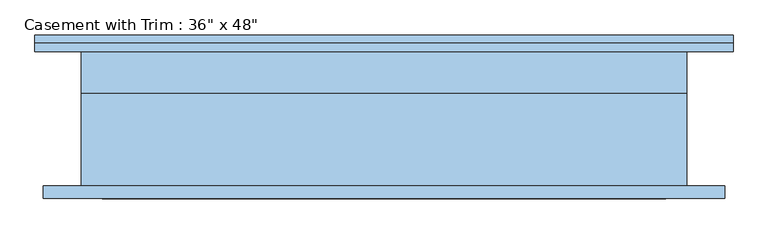
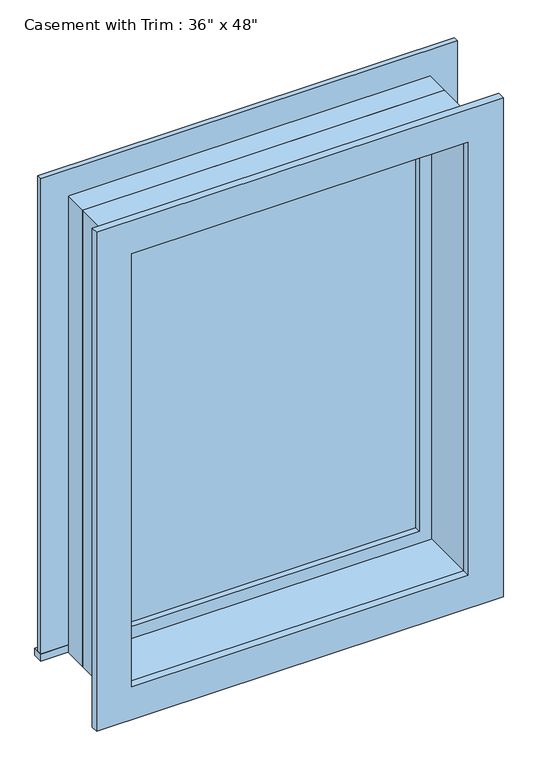
"""IFC4 building model written with IfcOpenShell, lengths in millimetres: window geometry."""

from ifc_helpers import new_model, si_unit, frame, origin, place, context, project, spatial, polyline, outline, extrude, source, transform, mapped, element, save


def window_8a4441b2(model_context):
    return source(origin(), model_context, "Body", "SweptSolid", [
        extrude(outline(polyline([(-527.05, 127.0), (527.05, 127.0), (527.05, 101.6), (-527.05, 101.6), (-527.05, 127.0)])), frame((0.0, 0.0, 914.4), z_axis=(0.0, 0.0, 1.0), x_axis=(1.0, 0.0, 0.0)), (0.0, 0.0, 1.0), 19.05),
        extrude(outline(polyline([(2114.55, -438.15), (2114.55, 438.15), (933.45, 438.15), (933.45, 527.05), (2203.45, 527.05), (2203.45, -527.05), (933.45, -527.05), (933.45, -438.15), (2114.55, -438.15)])), frame((0.0, 101.6, 0.0), z_axis=(0.0, 1.0, 0.0), x_axis=(0.0, 0.0, 1.0)), (0.0, 0.0, 1.0), 12.7),
        extrude(outline(polyline([(2190.75, 514.35), (2190.75, -514.35), (857.25, -514.35), (857.25, 514.35), (2190.75, 514.35)]), holes=[polyline([(2101.85, 425.45), (946.15, 425.45), (946.15, -425.45), (2101.85, -425.45), (2101.85, 425.45)])]), frame((0.0, -120.65, 0.0), z_axis=(0.0, 1.0, 0.0), x_axis=(0.0, 0.0, 1.0)), (0.0, 0.0, 1.0), 19.05),
        extrude(outline(polyline([(393.7, 53.975), (-393.7, 53.975), (-393.7, 66.675), (393.7, 66.675), (393.7, 53.975)])), frame((0.0, 0.0, 977.9), z_axis=(0.0, 0.0, 1.0), x_axis=(1.0, 0.0, 0.0)), (0.0, 0.0, 1.0), 1092.2),
        extrude(outline(polyline([(2114.55, -438.15), (933.45, -438.15), (933.45, 438.15), (2114.55, 438.15), (2114.55, -438.15)]), holes=[polyline([(2070.1, -393.7), (2070.1, 393.7), (977.9, 393.7), (977.9, -393.7), (2070.1, -393.7)])]), frame((0.0, 38.1, 0.0), z_axis=(0.0, 1.0, 0.0), x_axis=(0.0, 0.0, 1.0)), (0.0, 0.0, 1.0), 44.45),
        extrude(outline(polyline([(2133.6, -457.2), (914.4, -457.2), (914.4, 457.2), (2133.6, 457.2), (2133.6, -457.2)]), holes=[polyline([(2101.85, -425.45), (2101.85, 425.45), (946.15, 425.45), (946.15, -425.45), (2101.85, -425.45)])]), frame((0.0, -101.6, 0.0), z_axis=(0.0, 1.0, 0.0), x_axis=(0.0, 0.0, 1.0)), (0.0, 0.0, 1.0), 139.7),
        extrude(outline(polyline([(2133.6, 457.2), (2133.6, -457.2), (914.4, -457.2), (914.4, 457.2), (2133.6, 457.2)]), holes=[polyline([(2114.55, 438.15), (933.45, 438.15), (933.45, -438.15), (2114.55, -438.15), (2114.55, 438.15)])]), frame((0.0, 38.1, 0.0), z_axis=(0.0, 1.0, 0.0), x_axis=(0.0, 0.0, 1.0)), (0.0, 0.0, 1.0), 63.5),
    ])


if __name__ == "__main__":
    model = new_model("IFC4")
    model_context = context("Model", 3, world=origin())
    ifc_project = project(units=[si_unit("LENGTHUNIT", "METRE", prefix="MILLI")], contexts=[model_context])
    site = spatial("IfcSite", under=ifc_project)
    building = spatial("IfcBuilding", under=site)
    placement = place(None, origin())
    window_shape = window_8a4441b2(model_context)
    element("IfcWindow", 1, ObjectType="Casement with Trim : 36\" x 48\"", at=placement, inside=building, context=model_context, shape_type="MappedRepresentation", body=[
        mapped(window_shape, transform((0.0, 0.0, 0.0), x_axis=(1.0, 0.0, 0.0), y_axis=(0.0, 1.0, 0.0), z_axis=(0.0, 0.0, 1.0))),
    ])
    save(model, "model.ifc")

# Revit data of these elements
# Type "Casement with Trim : 36\" x 48\""
#   Type Mark = "14"
#   Construction Type Id = "GSP4R"
#   Assembly Code = "B2020100"
#   Analytic Construction = "1/8 in Pilkington single glazing"
#   Visual Light Transmittance = 0.9
#   Solar Heat Gain Coefficient = 0.78
#   Heat Transfer Coefficient (U) = 0.6496 BTU/(h·ft²·°F)
#   Height = 4' - 0"
#   Default Sill Height = 3' - 0"
#   Trim Projection - Ext. = 0' - 0 1/2"
#   Trim Projection - Int. = 0' - 0 3/4"
#   Trim Width - Exterior = 0' - 3 1/2"
#   Trim Width - Interior = 0' - 3 1/2"
#   Width = 3' - 0"
#   Window Inset = 0' - 0 3/4"
#   Define Thermal Properties by = 1
#   Glass Pane Material = Glass
#   Sash Material = Sash
#   Trim Exterior Material = Trim
#   Trim Interior Material = Trim
#   Wall Closure = (empty or 0)
# Element 1 (IfcWindow, "Casement with Trim : 36\" x 48\"")
#   Materials on its faces: "Sash", "Trim", "Glass"
# Materials
#   "Glass": class "Glass", colour RGB 0 128 192, transparency 0.75, Description = "Soda Lime Glass", Cost = 0
#   "Sash": class "Wood", colour RGB 224 178 126, transparency 0
#   "Trim": class "Wood", colour RGB 224 178 126, transparency 0
